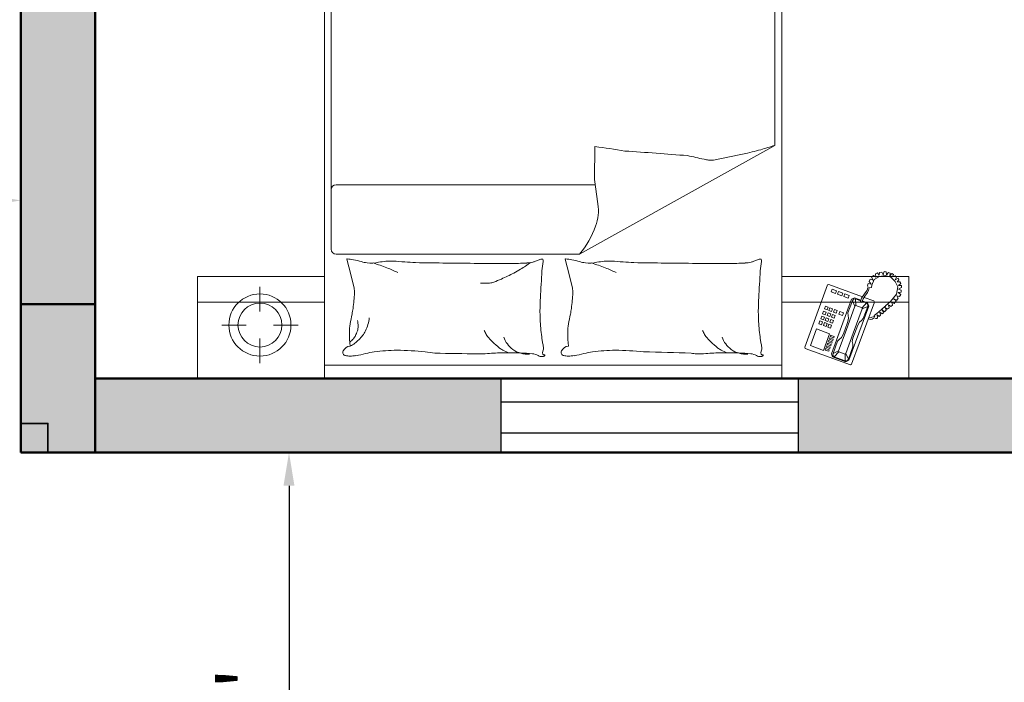
# Model space of a CAD drawing. Units: inches. Extents: x -7 to 1228, y -146 to 1091.
# Tile 3 of 88: x 60 to 179, y 32 to 112. Entities that reach past the tile are written whole.
import ezdxf

# ---------------------------------------------------------------- set-up
doc = ezdxf.new("R2010")
doc.units = ezdxf.units.IN
for name, color, linetype, lineweight in [('A-ANNO-DIMS', 2, 'Continuous', 18), ('A-COLS', 6, 'Continuous', 35), ('A-FURN', 8, 'Continuous', 18), ('A-GLAZ', 175, 'Continuous', 25), ('A-WALL', 7, 'Continuous', 50), ('A-WALL-PATT', 251, 'Continuous', 13)]:
    doc.layers.add(name, color=color, linetype=linetype, lineweight=lineweight)
doc.styles.add('DIM_FONT', font='SIMPLEX.shx', dxfattribs={"width": 0.8})
doc.styles.get("Standard").update_dxf_attribs({"font": 'arial.ttf'})
doc.dimstyles.new('ISO-25', dxfattribs={"dimtxt": 7, "dimasz": 4, "dimexe": 1.25, "dimexo": 0.625, "dimtad": 1, "dimdec": 1, "dimlunit": 3, "dimtxsty": 'Standard', "dimcen": 2.5, "dimadec": 0, "dimazin": 0, "dimtfac": 1, "dimtdec": 1, "dimtmove": 1, "dimatfit": 3, "dimfxl": 1, "dimarcsym": 0})

# ---------------------------------------------------------------- blocks, each defined once
blk = doc.blocks.new('A$C4F634EDD')
for p, q in [((0, 2.6295), (0, 2.2295)), ((0.5, 2.6295), (0, 2.6295)), ((0.5, 2.6295), (2.3, 2.6295)), ((0.5, 0.5295), (0.5, 2.6295)), ((0.5, 2.2295), (0.5, 2.6295)), ((2.3, 2.6295), (2.3, 0.5295)), ((2.3, 2.6295), (2.8, 2.6295)), ((2.3, 2.2295), (2.3, 2.6295)), ((2.8, 2.6295), (2.8, 2.2295)), ((0.2457, 2.5697), (0.2457, 2.4733)), ((0.5, 2.5771), (2.3, 2.5771)), ((2.392, 2.5115), (2.5692, 2.5765)), ((2.4985, 2.5445), (2.5516, 2.564)), ((2.5062, 2.5454), (2.5487, 2.561)), ((2.5483, 2.5347), (2.5487, 2.561)), ((2.5487, 2.561), (2.5571, 2.56)), ((2.5516, 2.564), (2.5637, 2.5584)), ((2.5571, 2.56), (2.5615, 2.5536)), ((2.5637, 2.5584), (2.6418, 2.3458)), ((2.5692, 2.5765), (2.574, 2.5743)), ((2.574, 2.5743), (2.6638, 2.3298)), ((2.412, 2.5007), (2.4634, 2.5196)), ((2.4634, 2.5196), (2.4875, 2.454)), ((2.4842, 2.5232), (2.47, 2.518)), ((2.4862, 2.5179), (2.4842, 2.5232)), ((2.4946, 2.5331), (2.4985, 2.5445)), ((2.5734, 2.3187), (2.4946, 2.5331)), ((2.5062, 2.5454), (2.5004, 2.5392)), ((2.5004, 2.5392), (2.5013, 2.5315)), ((2.5013, 2.5315), (2.5188, 2.4836)), ((2.5013, 2.5315), (2.5231, 2.5214)), ((2.5235, 2.5256), (2.5062, 2.5454)), ((2.5231, 2.5214), (2.5235, 2.5256)), ((2.5523, 2.4417), (2.5231, 2.5214)), ((2.5483, 2.5347), (2.5235, 2.5256)), ((2.5514, 2.5318), (2.5483, 2.5347)), ((2.5615, 2.5536), (2.5514, 2.5318)), ((2.5807, 2.4521), (2.5514, 2.5318)), ((2.5615, 2.5536), (2.5791, 2.5058)), ((2.3898, 2.5066), (2.392, 2.5115)), ((2.4795, 2.2621), (2.3898, 2.5066)), ((2.4361, 2.4352), (2.412, 2.5007)), ((2.47, 2.518), (2.472, 2.5127)), ((2.472, 2.5127), (2.4862, 2.5179)), ((2.4881, 2.5126), (2.4739, 2.5074)), ((2.4739, 2.5074), (2.4759, 2.502)), ((2.4759, 2.502), (2.4901, 2.5073)), ((2.492, 2.5019), (2.4778, 2.4967)), ((2.4778, 2.4967), (2.4798, 2.4914)), ((2.4798, 2.4914), (2.494, 2.4966)), ((2.4959, 2.4913), (2.4817, 2.4861)), ((2.4817, 2.4861), (2.4837, 2.4808)), ((2.4837, 2.4808), (2.4979, 2.486)), ((2.4998, 2.4807), (2.4856, 2.4755)), ((2.4901, 2.5073), (2.4881, 2.5126)), ((2.494, 2.4966), (2.492, 2.5019)), ((2.4979, 2.486), (2.4959, 2.4913)), ((2.5018, 2.4754), (2.4998, 2.4807)), ((2.5188, 2.4836), (2.5256, 2.4761)), ((2.5788, 2.4956), (2.5767, 2.4848)), ((2.5767, 2.4848), (2.5795, 2.4717)), ((2.5791, 2.5058), (2.5788, 2.4956)), ((2.4875, 2.454), (2.4361, 2.4352)), ((2.4856, 2.4755), (2.4876, 2.4702)), ((2.4876, 2.4702), (2.5018, 2.4754)), ((2.5037, 2.47), (2.4895, 2.4648)), ((2.4895, 2.4648), (2.4915, 2.4595)), ((2.4915, 2.4595), (2.5057, 2.4647)), ((2.5057, 2.4647), (2.5037, 2.47)), ((2.5256, 2.4761), (2.5342, 2.4692)), ((2.5342, 2.4692), (2.5405, 2.4574)), ((2.5405, 2.4574), (2.547, 2.4397)), ((2.5523, 2.4417), (2.5875, 2.346)), ((2.5795, 2.4717), (2.586, 2.454)), ((2.5807, 2.4521), (2.6158, 2.3564)), ((2.5984, 2.4204), (2.586, 2.454)), ((0.0957, 2.4197), (0.192, 2.4197)), ((0.2994, 2.4197), (0.3957, 2.4197)), ((2.4457, 2.4146), (2.4563, 2.4185)), ((2.4496, 2.4039), (2.4457, 2.4146)), ((2.4602, 2.4078), (2.4496, 2.4039)), ((2.4563, 2.4185), (2.4602, 2.4078)), ((2.4634, 2.4211), (2.474, 2.425)), ((2.4673, 2.4104), (2.4634, 2.4211)), ((2.4779, 2.4143), (2.4673, 2.4104)), ((2.4706, 2.4016), (2.4812, 2.4055)), ((2.474, 2.425), (2.4779, 2.4143)), ((2.4811, 2.4276), (2.4917, 2.4315)), ((2.485, 2.4169), (2.4811, 2.4276)), ((2.4812, 2.4055), (2.4851, 2.3949)), ((2.4956, 2.4208), (2.485, 2.4169)), ((2.4883, 2.4081), (2.4989, 2.412)), ((2.4922, 2.3975), (2.4883, 2.4081)), ((2.4917, 2.4315), (2.4956, 2.4208)), ((2.4989, 2.412), (2.5028, 2.4014)), ((2.5594, 2.4061), (2.547, 2.4397)), ((2.5622, 2.393), (2.5594, 2.4061)), ((2.6047, 2.4086), (2.5984, 2.4204)), ((2.6133, 2.4017), (2.6047, 2.4086)), ((0.2457, 2.366), (0.2457, 2.2697)), ((2.4528, 2.3951), (2.4635, 2.399)), ((2.4567, 2.3844), (2.4528, 2.3951)), ((2.4674, 2.3883), (2.4567, 2.3844)), ((2.46, 2.3756), (2.4706, 2.3795)), ((2.4639, 2.365), (2.46, 2.3756)), ((2.4635, 2.399), (2.4674, 2.3883)), ((2.4745, 2.3689), (2.4639, 2.365)), ((2.4745, 2.3909), (2.4706, 2.4016)), ((2.4706, 2.3795), (2.4745, 2.3689)), ((2.4851, 2.3949), (2.4745, 2.3909)), ((2.4777, 2.3821), (2.4883, 2.386)), ((2.4816, 2.3715), (2.4777, 2.3821)), ((2.4922, 2.3754), (2.4816, 2.3715)), ((2.4849, 2.3626), (2.4955, 2.3665)), ((2.4883, 2.386), (2.4922, 2.3754)), ((2.5028, 2.4014), (2.4922, 2.3975)), ((2.4954, 2.3886), (2.5061, 2.3925)), ((2.4993, 2.378), (2.4954, 2.3886)), ((2.4955, 2.3665), (2.4994, 2.3559)), ((2.51, 2.3819), (2.4993, 2.378)), ((2.5026, 2.3691), (2.5132, 2.373)), ((2.5065, 2.3585), (2.5026, 2.3691)), ((2.5061, 2.3925), (2.51, 2.3819)), ((2.5132, 2.373), (2.5171, 2.3624)), ((2.5238, 2.3769), (2.538, 2.3821)), ((2.5277, 2.3663), (2.5238, 2.3769)), ((2.5419, 2.3715), (2.5277, 2.3663)), ((2.538, 2.3821), (2.5419, 2.3715)), ((2.5598, 2.372), (2.5601, 2.3822)), ((2.5774, 2.3242), (2.5598, 2.372)), ((2.5601, 2.3822), (2.5622, 2.393)), ((2.6201, 2.3941), (2.6133, 2.4017)), ((2.6376, 2.3463), (2.6201, 2.3941)), ((2.6499, 2.3979), (2.6397, 2.3953)), ((2.6417, 2.39), (2.6488, 2.391)), ((2.6488, 2.391), (2.6538, 2.3895)), ((2.6551, 2.397), (2.6499, 2.3979)), ((2.6538, 2.3895), (2.6596, 2.388)), ((2.6627, 2.392), (2.6551, 2.397)), ((2.6596, 2.388), (2.6626, 2.3867)), ((2.6626, 2.3867), (2.6662, 2.388)), ((2.6692, 2.394), (2.6627, 2.392)), ((2.6662, 2.388), (2.6632, 2.3828)), ((2.6632, 2.3828), (2.6736, 2.3744)), ((2.6736, 2.3944), (2.6692, 2.394)), ((2.6765, 2.391), (2.6736, 2.3944)), ((2.6736, 2.3744), (2.6922, 2.3593)), ((2.6742, 2.3795), (2.6765, 2.391)), ((2.6824, 2.3858), (2.6742, 2.3795)), ((2.6873, 2.3815), (2.6824, 2.3858)), ((2.6853, 2.369), (2.6873, 2.3815)), ((2.6946, 2.376), (2.6853, 2.369)), ((2.6995, 2.3713), (2.6946, 2.376)), ((2.695, 2.3603), (2.6995, 2.3713)), ((2.7031, 2.3682), (2.695, 2.3603)), ((2.7096, 2.3616), (2.7031, 2.3682)), ((0, 2.3301), (0.5, 2.3301)), ((2.8, 2.3301), (2.3, 2.3301)), ((2.4672, 2.3561), (2.4778, 2.36)), ((2.4711, 2.3455), (2.4672, 2.3561)), ((2.4817, 2.3494), (2.4711, 2.3455)), ((2.4778, 2.36), (2.4817, 2.3494)), ((2.4888, 2.352), (2.4849, 2.3626)), ((2.4994, 2.3559), (2.4888, 2.352)), ((2.5171, 2.3624), (2.5065, 2.3585)), ((2.5774, 2.3242), (2.5875, 2.346)), ((2.5875, 2.346), (2.5905, 2.3431)), ((2.5905, 2.3431), (2.5901, 2.3168)), ((2.6154, 2.3522), (2.5905, 2.3431)), ((2.613, 2.3312), (2.6077, 2.3293)), ((2.6077, 2.3293), (2.6135, 2.3141)), ((2.6192, 2.3174), (2.613, 2.3312)), ((2.6153, 2.3261), (2.6327, 2.3324)), ((2.6158, 2.3564), (2.6154, 2.3522)), ((2.6154, 2.3522), (2.6327, 2.3324)), ((2.6376, 2.3463), (2.6158, 2.3564)), ((2.6369, 2.332), (2.6161, 2.3243)), ((2.6616, 2.3249), (2.6234, 2.3109)), ((2.6327, 2.3324), (2.6385, 2.3386)), ((2.6418, 2.3458), (2.6369, 2.332)), ((2.6385, 2.3386), (2.6376, 2.3463)), ((2.6638, 2.3298), (2.6616, 2.3249)), ((2.6922, 2.3593), (2.7051, 2.3473)), ((2.7051, 2.3473), (2.7079, 2.3475)), ((2.7062, 2.351), (2.7096, 2.3616)), ((2.7147, 2.3578), (2.7062, 2.351)), ((2.7079, 2.3475), (2.7079, 2.3443)), ((2.7079, 2.3443), (2.727, 2.3277)), ((2.7214, 2.3517), (2.7147, 2.3578)), ((2.7196, 2.34), (2.7214, 2.3517)), ((2.7286, 2.3466), (2.7196, 2.34)), ((2.727, 2.3277), (2.7512, 2.2983)), ((2.7346, 2.3423), (2.7286, 2.3466)), ((2.732, 2.3295), (2.7346, 2.3423)), ((2.7423, 2.3345), (2.732, 2.3295)), ((2.7406, 2.3172), (2.7495, 2.325)), ((2.7495, 2.325), (2.7423, 2.3345)), ((2.6172, 2.3086), (2.4844, 2.2599)), ((2.5114, 2.2959), (2.4936, 2.2894)), ((2.4936, 2.2894), (2.4976, 2.2788)), ((2.5153, 2.2853), (2.5114, 2.2959)), ((2.5362, 2.305), (2.5185, 2.2985)), ((2.5185, 2.2985), (2.5224, 2.2879)), ((2.5224, 2.2879), (2.5401, 2.2944)), ((2.5401, 2.2944), (2.5362, 2.305)), ((2.561, 2.3141), (2.5433, 2.3076)), ((2.5433, 2.3076), (2.5472, 2.297)), ((2.5472, 2.297), (2.5649, 2.3035)), ((2.5649, 2.3035), (2.561, 2.3141)), ((2.5855, 2.3131), (2.5734, 2.3187)), ((2.5818, 2.3178), (2.5774, 2.3242)), ((2.5901, 2.3168), (2.5818, 2.3178)), ((2.6104, 2.3222), (2.5855, 2.3131)), ((2.5901, 2.3168), (2.6097, 2.324)), ((2.6135, 2.3141), (2.6244, 2.2977)), ((2.626, 2.3069), (2.6192, 2.3174)), ((2.6244, 2.2977), (2.6349, 2.2825)), ((2.6365, 2.2916), (2.626, 2.3069)), ((2.6407, 2.2834), (2.6365, 2.2916)), ((2.7519, 2.3218), (2.7406, 2.3172)), ((2.7512, 2.2983), (2.756, 2.2695)), ((2.7575, 2.3144), (2.7519, 2.3218)), ((2.7526, 2.3045), (2.7575, 2.3144)), ((2.7622, 2.308), (2.7526, 2.3045)), ((2.7574, 2.2924), (2.7673, 2.2997)), ((2.7687, 2.2905), (2.7574, 2.2924)), ((2.7673, 2.2997), (2.7622, 2.308)), ((2.7699, 2.2828), (2.7687, 2.2905)), ((0.5953, 2.1912), (0.616, 2.2738)), ((1.4546, 2.1912), (1.4752, 2.2738)), ((2.4844, 2.2599), (2.4795, 2.2621)), ((2.4976, 2.2788), (2.5153, 2.2853)), ((2.6349, 2.2825), (2.638, 2.273)), ((2.6399, 2.2712), (2.6374, 2.2659)), ((2.6374, 2.2659), (2.6398, 2.257)), ((2.638, 2.273), (2.6399, 2.2712)), ((2.6398, 2.257), (2.6509, 2.259)), ((2.6438, 2.2739), (2.6407, 2.2834)), ((2.6509, 2.259), (2.6431, 2.2492)), ((2.6431, 2.2492), (2.6473, 2.2398)), ((2.6519, 2.2716), (2.6438, 2.2739)), ((2.6535, 2.2628), (2.6519, 2.2716)), ((2.6636, 2.2409), (2.6535, 2.2628)), ((2.7459, 2.2483), (2.7284, 2.2317)), ((2.756, 2.2695), (2.7459, 2.2483)), ((2.7529, 2.2505), (2.7645, 2.2498)), ((2.7607, 2.2424), (2.7529, 2.2505)), ((2.7587, 2.279), (2.7699, 2.2828)), ((2.7708, 2.2725), (2.7587, 2.279)), ((2.759, 2.2637), (2.7706, 2.2643)), ((2.7676, 2.2559), (2.759, 2.2637)), ((2.7645, 2.2498), (2.7676, 2.2559)), ((2.7706, 2.2643), (2.7708, 2.2725)), ((0, 2.2295), (0.5, 2.2295)), ((2.8, 2.2295), (2.3, 2.2295)), ((2.6473, 2.2398), (2.6592, 2.2429)), ((2.6592, 2.2429), (2.6521, 2.2314)), ((2.6521, 2.2314), (2.6598, 2.2248)), ((2.6598, 2.2248), (2.6697, 2.2309)), ((2.6836, 2.2287), (2.6636, 2.2409)), ((2.6697, 2.2309), (2.6684, 2.219)), ((2.6684, 2.219), (2.6761, 2.2145)), ((2.6761, 2.2145), (2.6821, 2.2237)), ((2.6821, 2.2237), (2.6843, 2.2135)), ((2.7063, 2.2256), (2.6836, 2.2287)), ((2.6843, 2.2135), (2.6927, 2.2117)), ((2.6927, 2.2117), (2.6986, 2.222)), ((2.6986, 2.222), (2.7019, 2.2098)), ((2.7019, 2.2098), (2.7102, 2.2104)), ((2.7284, 2.2317), (2.7063, 2.2256)), ((2.7102, 2.2104), (2.7113, 2.2218)), ((2.7113, 2.2218), (2.7192, 2.2137)), ((2.7192, 2.2137), (2.7255, 2.2152)), ((2.7255, 2.2152), (2.7242, 2.2265)), ((2.7242, 2.2265), (2.7324, 2.2165)), ((2.7324, 2.2165), (2.7386, 2.2208)), ((2.7386, 2.2208), (2.7354, 2.2306)), ((2.7354, 2.2306), (2.7462, 2.2264)), ((2.7509, 2.2314), (2.7459, 2.2418)), ((2.7459, 2.2418), (2.7568, 2.2352)), ((2.7462, 2.2264), (2.7509, 2.2314)), ((2.7568, 2.2352), (2.7607, 2.2424)), ((0.5878, 2.1612), (0.5953, 2.1912)), ((1.4471, 2.1612), (1.4546, 2.1912)), ((1.5035, 2.141), (0.5458, 2.141)), ((1.5035, 2.141), (2.2716, 1.7136)), ((0.5258, 2.121), (0.5258, 0.5617)), ((1.576, 1.9433), (1.5624, 1.8479)), ((0.5458, 1.8684), (1.5653, 1.8684)), ((1.5624, 1.8479), (1.5641, 1.7178)), ((2.2716, 0.5617), (2.2716, 1.7136))]:
    blk.add_line(p, q)
for radius in [0.1222, 0.0865]:
    blk.add_circle((0.2457, 2.4197), radius)
for centre, radius, start, end in [((0.5848, 2.5274), 0.0131, 101.2724, 206.5805), ((0.6036, 2.5368), 0.0342, 206.5805, 265.5998), ((0.5999, 2.4516), 0.0904, 90, 101.2724), ((0.5999, 2.3808), 0.1611, 81.5628, 90), ((0.5788, 2.2388), 0.3048, 74.256, 81.5628), ((0.7272, 2.7653), 0.2422, 254.256, 262.4531), ((0.7851, 3.2019), 0.6827, 262.4531, 270), ((0.7851, 3.5682), 1.049, 270, 276.0867), ((0.8402, 3.0514), 0.5293, 276.0867, 280.1899), ((1.1602, -8.1346), 10.6675, 90.30153, 91.21582), ((1.1169, 2.2433), 0.2897, 85.1982, 92.5386), ((1.2142, 3.4021), 0.8732, 265.1982, 269.4243), ((1.3082, 2.3102), 0.234, 110.8603, 117.2396), ((1.2204, 4.0232), 1.4943, 269.4243, 271.9079), ((1.2995, 2.4357), 0.0992, 105.9352, 126.0864), ((1.2429, 3.3501), 0.8208, 271.9079, 275.2592), ((1.2995, 2.4357), 0.0992, 85.7841, 105.9352), ((1.3132, 2.5864), 0.0539, 275.2592, 300.6513), ((1.3554, 2.5152), 0.0289, 85.6975, 120.6513), ((1.3556, 2.519), 0.0251, 68.2117, 85.6975), ((1.3739, 2.5288), 0.0156, 158.0096, 201.421), ((1.3634, 2.533), 0.00428, 78.1069, 158.0096), ((1.3288, 2.5111), 0.0328, 351.8665, 21.421), ((1.3647, 2.5395), 0.00232, 258.1069, 19.564), ((1.3637, 2.5391), 0.00342, 19.564, 68.2117), ((1.444, 2.5274), 0.0131, 101.2724, 206.5805), ((1.4628, 2.5368), 0.0342, 206.5805, 265.5998), ((1.4591, 2.4516), 0.0904, 90, 101.2724), ((1.4591, 2.3808), 0.1611, 81.5628, 90), ((1.438, 2.2388), 0.3048, 74.256, 81.5628), ((1.5865, 2.7653), 0.2422, 254.256, 262.4531), ((1.6443, 3.2019), 0.6827, 262.4531, 270), ((1.6443, 3.5682), 1.049, 270, 276.0867), ((1.4785, 15.4878), 12.9656, 271.22425, 272.05324), ((1.97, 2.3805), 0.1524, 92.5386, 100.1899), ((1.9761, 2.2433), 0.2897, 85.1982, 92.5386), ((2.0734, 3.4021), 0.8732, 265.1982, 269.4243), ((2.1674, 2.3102), 0.234, 110.8603, 117.2396), ((2.0797, 4.0232), 1.4943, 269.4243, 271.9079), ((2.1588, 2.4357), 0.0992, 105.9352, 126.0864), ((2.1021, 3.3501), 0.8208, 271.9079, 275.2592), ((2.1588, 2.4357), 0.0992, 85.7841, 105.9352), ((2.1724, 2.5864), 0.0539, 275.2592, 300.6513), ((2.2146, 2.5152), 0.0289, 85.6975, 120.6513), ((2.2149, 2.519), 0.0251, 68.2117, 85.6975), ((2.2331, 2.5288), 0.0156, 158.0096, 201.421), ((2.2226, 2.533), 0.00428, 78.1069, 158.0096), ((2.1881, 2.5111), 0.0328, 351.8665, 21.421), ((2.224, 2.5395), 0.00232, 258.1069, 19.564), ((2.2229, 2.5391), 0.00342, 19.564, 68.2117), ((1.0898, 2.4496), 0.4918, 173.7676, 180), ((0.5462, 2.4142), 0.0899, 41.4429, 53.7359), ((0.5368, 2.3783), 0.1399, 45.0976, 62.7964), ((1.3165, 2.3233), 0.2252, 133.8115, 140.9651), ((1.4317, 2.2032), 0.3916, 128.3886, 133.8115), ((1.2362, 2.45), 0.0768, 117.2396, 128.3886), ((1.2995, 2.4357), 0.0992, 143.8234, 161.5603), ((1.2995, 2.4357), 0.0992, 126.0864, 143.8234), ((1.5522, 2.448), 0.1983, 167.8905, 172.3191), ((1.1177, 2.5413), 0.246, 347.8905, 351.8665), ((1.949, 2.4496), 0.4918, 173.7676, 180), ((2.1757, 2.3233), 0.2252, 133.8115, 140.9651), ((2.291, 2.2032), 0.3916, 128.3886, 133.8115), ((2.0954, 2.45), 0.0768, 117.2396, 128.3886), ((2.1588, 2.4357), 0.0992, 143.8234, 161.5603), ((2.1588, 2.4357), 0.0992, 126.0864, 143.8234), ((2.4114, 2.448), 0.1983, 167.8905, 172.3191), ((1.977, 2.5413), 0.246, 347.8905, 351.8665), ((0.8019, 2.4496), 0.204, 180, 189.6844), ((0.5741, 2.4389), 0.0526, 25.3551, 41.4429), ((0.4851, 2.3967), 0.1511, 21.8149, 25.3551), ((0.4345, 2.3765), 0.2056, 18.7799, 21.8149), ((0.576, 2.4246), 0.0562, 0, 18.7799), ((0.5368, 2.3783), 0.1399, 27.3988, 45.0976), ((0.5368, 2.3783), 0.1399, 16.515, 27.3988), ((1.3127, 2.3625), 0.2002, 151.6832, 156.9972), ((1.1799, 2.4341), 0.0493, 140.9651, 151.6832), ((2.2605, 2.3525), 0.9131, 172.3191, 176.6313), ((1.6611, 2.4496), 0.204, 180, 189.6844), ((2.1719, 2.3625), 0.2002, 151.6832, 156.9972), ((2.0391, 2.4341), 0.0493, 140.9651, 151.6832), ((3.1198, 2.3525), 0.9131, 172.3191, 176.6313), ((1.4703, 2.5637), 0.882, 189.6844, 192.1984), ((0.5406, 2.4246), 0.0915, 345.3149, 0), ((0.5368, 2.3783), 0.1399, 5.6311, 16.515), ((2.0266, 2.3663), 0.6787, 176.6313, 181.6331), ((2.3295, 2.5637), 0.882, 189.6844, 192.1984), ((2.8858, 2.3663), 0.6787, 176.6313, 181.6331), ((0.2982, 2.3103), 0.3171, 8.0051, 12.1984), ((1.1575, 2.3103), 0.3171, 8.0051, 12.1984), ((-0.0401, 2.2627), 0.6588, 2.6649, 8.0051), ((2.7128, 2.3859), 1.3652, 181.6331, 183.055), ((0.8191, 2.2627), 0.6588, 2.6649, 8.0051), ((3.5721, 2.3859), 1.3652, 181.6331, 183.055), ((0.5503, 2.2902), 0.0677, 345.9548, 2.6649), ((14.9657, 3.0398), 13.6356, 183.05496, 183.50486), ((1.4096, 2.2902), 0.0677, 345.9548, 2.6649), ((15.8249, 3.0398), 13.6356, 183.05496, 183.50486), ((1.1303, 1.9835), 0.2721, 85.9172, 93.5552), ((1.1455, 2.197), 0.058, 69.3257, 85.9172), ((0.9871, 1.7772), 0.5066, 65.6735, 69.3257), ((0.473, 2.8815), 0.7387, 293.4844, 295.3111), ((0.6058, 0.9338), 1.4323, 63.5015, 65.6735), ((1.1054, 1.9358), 0.3126, 57.865, 63.5015), ((1.3322, 2.8815), 0.7387, 293.4844, 295.3111), ((0.5763, 2.3896), 0.2297, 279.4841, 287.3864), ((0.6807, 2.0561), 0.1197, 96.4341, 107.3864), ((0.6836, 2.0301), 0.1459, 78.4414, 96.4341), ((0.473, 2.8815), 0.7387, 287.1982, 289.428), ((0.759, 2.3985), 0.2301, 258.4414, 272.7491), ((0.473, 2.8815), 0.7387, 289.428, 291.6577), ((0.473, 2.8815), 0.7387, 291.6577, 293.4844), ((0.7026, 3.5718), 1.4048, 272.7491, 274.6176), ((0.9136, 0.9591), 1.2165, 92.6096, 94.6176), ((1.2501, -19.8405), 22.0183, 90.37908, 91.01965), ((1.2012, -3.5404), 5.7185, 89.7135, 90.9704), ((1.224, 1.0141), 1.164, 86.426, 89.7135), ((0.8841, 1.5835), 0.7286, 54.1737, 57.865), ((1.2875, 2.0302), 0.1459, 77.131, 86.426), ((1.3099, 2.1283), 0.0453, 62.7159, 77.131), ((1.6762, 2.2258), 0.3212, 183.5049, 189.9984), ((1.3409, 2.1667), 0.0193, 343.3022, 9.9984), ((1.4355, 2.3896), 0.2297, 279.4841, 287.3864), ((1.5399, 2.0561), 0.1197, 96.4341, 107.3864), ((1.5429, 2.0301), 0.1459, 78.4414, 96.4341), ((1.3322, 2.8815), 0.7387, 287.1982, 289.428), ((1.6182, 2.3985), 0.2301, 258.4414, 272.7491), ((1.3322, 2.8815), 0.7387, 289.428, 291.6577), ((1.3322, 2.8815), 0.7387, 291.6577, 293.4844), ((1.5619, 3.5718), 1.4048, 272.7491, 274.6176), ((1.7729, 0.9591), 1.2165, 92.6096, 94.6176), ((2.1093, -19.8405), 22.0183, 90.37908, 91.01965), ((2.0605, -3.5404), 5.7185, 89.7135, 90.9704), ((2.0833, 1.0141), 1.164, 86.426, 89.7135), ((2.1467, 2.0302), 0.1459, 77.131, 86.426), ((2.1691, 2.1283), 0.0453, 62.7159, 77.131), ((2.5355, 2.2258), 0.3212, 183.5049, 189.9984), ((2.2001, 2.1667), 0.0193, 343.3022, 9.9984), ((0.5458, 2.121), 0.02, 90, 180), ((0.5887, 2.1609), 0.000917, 165.9551, 274.0829), ((0.5695, 2.4301), 0.2708, 274.0829, 279.4841), ((1.3658, 2.2367), 0.0767, 242.7159, 253.7788), ((1.3688, 2.247), 0.0875, 253.7788, 262.8796), ((1.3581, 2.1615), 0.00132, 262.8796, 343.3022), ((1.448, 2.1609), 0.000917, 165.9551, 274.0829), ((1.4288, 2.4301), 0.2708, 274.0829, 279.4841), ((1.2147, 1.9017), 0.3751, 20.1488, 39.6445), ((2.2251, 2.2367), 0.0767, 242.7159, 253.7788), ((2.2281, 2.247), 0.0875, 253.7788, 262.8796), ((2.2174, 2.1615), 0.00132, 262.8796, 343.3022), ((1.3977, 1.9688), 0.1801, 351.8644, 20.1488), ((0.5458, 1.8884), 0.02, 180, 270), ((0.6102, 18.0525), 16.3521, 273.75703, 274.62393), ((1.4194, 4.2174), 2.5158, 281.6741, 283.1904), ((2.0378, 1.5789), 0.1942, 97.7304, 103.1904), ((2.0195, 1.7137), 0.0581, 79.2724, 97.7304), ((1.2737, -2.2227), 4.0646, 77.0745, 79.2724), ((1.0582, 5.4638), 3.7801, 277.692, 279.495), ((2.0359, 1.0981), 0.6574, 74.0648, 77.0745), ((1.7125, -0.0344), 1.8351, 72.2636, 74.0648)]:
    blk.add_arc(centre, radius, start, end)
at = {"style": 'DIM_FONT', "width": 0.8, "flags": 9}
for tag, p in [('YSIZE', (0.5, 2.6295)), ('XSIZE', (0.5, 2.6295)), ('XSIZE', (2.2985, 2.6295)), ('YSIZE', (2.2985, 2.6295))]:
    blk.add_attdef(tag, p, '', height=0.0005, dxfattribs=at)
blk = doc.blocks.new('*D9')
at = {"layer": 'A-ANNO-DIMS', "color": 0, "lineweight": -2, "transparency": 16777216}
for p, q in [((92.31, 60), (91.25, 60)), ((92.5, 56), (92.5, 4)), ((92.31, 0), (91.25, 0))]:
    blk.add_line(p, q, dxfattribs=at)
at = {"layer": 'A-ANNO-DIMS', "color": 0, "transparency": 16777216}
for points in [[(91.83, 56), (93.16, 56), (92.5, 60)], [(91.83, 4), (93.16, 4), (92.5, 0)]]:
    blk.add_solid(points, dxfattribs=at)
at = {"layer": 'Defpoints', "color": 0, "transparency": 16777216}
for p in [(92.94, 60), (92.94, 0), (92.5, 0)]:
    blk.add_point(p, dxfattribs=at)
at = {"layer": 'A-ANNO-DIMS', "color": 0, "transparency": 16777216, "insert": (88.31, 30), "char_height": 7, "attachment_point": 5, "rotation": 90}
blk.add_mtext("5'", dxfattribs=at)
blk = doc.blocks.new('*D10')
at = {"layer": 'A-ANNO-DIMS', "color": 0, "lineweight": -2, "transparency": 16777216}
for p, q in [((0, 96.81), (0, 89.3)), ((60, 96.81), (60, 89.3)), ((56, 90.55), (4, 90.55))]:
    blk.add_line(p, q, dxfattribs=at)
at = {"layer": 'A-ANNO-DIMS', "color": 0, "transparency": 16777216}
for points in [[(4, 91.22), (4, 89.88), (0, 90.55)], [(56, 91.22), (56, 89.88), (60, 90.55)]]:
    blk.add_solid(points, dxfattribs=at)
at = {"layer": 'Defpoints', "color": 0, "transparency": 16777216}
for p in [(0, 97.43), (60, 97.43), (0, 90.55)]:
    blk.add_point(p, dxfattribs=at)
at = {"layer": 'A-ANNO-DIMS', "color": 0, "transparency": 16777216, "insert": (30, 94.74), "char_height": 7, "attachment_point": 5}
blk.add_mtext("5'", dxfattribs=at)
blk = doc.blocks.new('WIN-36')
for p, q in [((0, 36), (0, 0)), ((9, 36), (0, 36)), ((2.34, 36), (2.34, 0)), ((6.14, 0), (6.14, 36)), ((9, 0), (9, 36)), ((0, 0), (9, 0)), ((2.34, 0), (6.14, 0))]:
    blk.add_line(p, q)

msp = doc.modelspace()

# ---------------------------------------------------------------- hatches: boundary and pattern name
at = {"layer": 'A-COLS'}
h = msp.add_hatch(color=256, dxfattribs=at)
h.dxf.hatch_style = 1
h.paths.add_polyline_path([(60, 63.55), (63.29, 63.55), (63.29, 60), (69, 60), (69, 78), (60, 78)])
h = msp.add_hatch(color=256, dxfattribs=at)
h.dxf.hatch_style = 1
h.paths.add_polyline_path([(60, 63.55), (60, 60), (63.29, 60), (63.29, 63.55)])
at = {"layer": 'A-WALL-PATT'}
h = msp.add_hatch(color=256, dxfattribs=at)
h.dxf.hatch_style = 1
h.paths.add_polyline_path([(69, 568), (60, 568), (60, 493), (63.29, 493), (69, 493)])
h.paths.add_polyline_path([(69, 662.41), (60, 662.41), (60, 586), (69, 586)], flags=17)
h.paths.add_polyline_path([(69, 723), (184, 723), (184, 734), (179, 734), (179, 728), (69, 728), (69, 741.62), (60, 741.62), (60, 698.41), (69, 698.41)], flags=17)
h.paths.add_polyline_path([(69, 782), (231, 782), (231, 728), (231, 723), (231, 586), (236, 586), (236, 787), (69, 787), (69, 800.13), (60, 800.13), (60, 765.62), (69, 765.62)])
h.paths.add_polyline_path([(184, 842), (189, 842), (189, 848), (173, 848), (173, 842), (179, 842), (179, 787), (184, 787)])
h.paths.add_polyline_path([(118.22, 69), (69, 69), (69, 60), (118.22, 60)])
h.paths.add_polyline_path([(227, 69), (154.22, 69), (154.22, 60), (227, 60)])
h.paths.add_polyline_path([(236, 60), (232.71, 60), (227, 60), (227, 36), (236, 36)])
h.paths.add_polyline_path([(389, 60), (380, 60), (380, 36), (389, 36)])
h.paths.add_polyline_path([(384, 181), (380, 181), (380, 115), (380, 78), (384, 78)])
h.paths.add_polyline_path([(380, 115), (334.55, 115), (334.55, 109), (380, 109)])
h.paths.add_polyline_path([(274.55, 115), (236, 115), (236, 201), (232.71, 201), (231, 201), (231, 78), (236, 78), (236, 109), (274.55, 109)])
h.paths.add_polyline_path([(69, 123), (60, 123), (60, 78), (69, 78)])
h.paths.add_polyline_path([(69, 201), (60, 201), (60, 159), (69, 159)])
h.paths.add_polyline_path([(143, 219), (69, 219), (69, 213), (143, 213)], flags=17)
h.paths.add_polyline_path([(189, 219), (184, 219), (184, 274), (231, 274), (231, 219), (236, 219), (236, 279), (184, 279), (184, 297), (179, 297), (179, 279), (69, 279), (69, 290.91), (60, 290.91), (60, 262.18), (69, 262.18), (69, 274), (179, 274), (179, 219), (173, 219), (173, 213), (189, 213)])
h.paths.add_polyline_path([(69, 238.18), (60, 238.18), (60, 219), (69, 219)], flags=17)
h.paths.add_polyline_path([(69, 333), (60, 333), (60, 314.91), (69, 314.91), (69, 316.96)])
h.paths.add_polyline_path([(190, 338), (184, 338), (69, 338), (69, 333), (179, 333), (179, 327), (184, 327), (184, 333.02), (190, 333.05)])
h.paths.add_polyline_path([(69, 386.81), (60, 386.81), (60, 351), (69, 351)])
h.paths.add_polyline_path([(69, 475), (60, 475), (60, 422.81), (69, 422.81)])
h.paths.add_polyline_path([(236, 475), (231, 475), (231, 351.24), (236, 351.24)])
h.paths.add_polyline_path([(384, 475), (380, 475), (380, 362), (384, 362)])
h.paths.add_polyline_path([(547, 307), (439, 307), (439, 356), (445, 356), (445, 362), (433, 362), (433, 307), (380, 307), (380, 244), (380, 241), (384, 241), (384, 301), (433, 301), (433, 277), (439, 277), (439, 301), (547, 301)])
h.paths.add_polyline_path([(547, 241), (439, 241), (439, 247), (433, 247), (433, 235), (547, 235)])
h.paths.add_polyline_path([(450, 69), (440.29, 69), (424.89, 69), (389, 69), (389, 60), (450, 60)])
h.paths.add_polyline_path([(547, 69), (486, 69), (486, 60), (547, 60)])
h.paths.add_polyline_path([(556, 148.27), (547, 148.27), (547, 78), (556, 78)])
h.paths.add_polyline_path([(556, 223), (547, 223), (547, 195), (547, 184.27), (556, 184.27)])
h.paths.add_polyline_path([(556, 311.19), (547, 311.19), (547, 273.08), (556, 273.08)])
h.paths.add_polyline_path([(556, 344), (552.71, 344), (547, 344), (547, 335.19), (556, 335.19)])
h.paths.add_polyline_path([(556, 249.08), (547, 249.08), (547, 241), (556, 241)])
h.paths.add_polyline_path([(547, 362), (475, 362), (475, 356), (547, 356)], flags=0)
h.paths.add_polyline_path([(556, 399.62), (547, 399.62), (547, 362), (556, 362)])
h.paths.add_polyline_path([(556, 475), (547, 475), (547, 435.62), (556, 435.62)])
h.paths.add_polyline_path([(547, 493), (389, 493), (389, 487), (547, 487)])
h.paths.add_polyline_path([(380, 493), (278, 493), (278, 487), (380, 487)])
h.paths.add_polyline_path([(227, 493), (69, 493), (69, 487), (227, 487)])
h.paths.add_polyline_path([(643, 122.44), (634, 122.44), (634, 78), (643, 78)])
h.paths.add_polyline_path([(702.5, 69), (692.79, 69), (677.39, 69), (643, 69), (643, 60), (702.5, 60)])
h.paths.add_polyline_path([(798, 69), (738.5, 69), (738.5, 60), (798, 60)])
h.paths.add_polyline_path([(807, 60), (803.71, 60), (798, 60), (798, 36), (807, 36)])
h.paths.add_polyline_path([(807, 109), (846.75, 109), (846.75, 115), (807, 115), (807, 159), (802, 159), (802, 78), (807, 78)])
h.paths.add_polyline_path([(807, 201), (802, 201), (802, 195), (807, 195)])
h.paths.add_polyline_path([(643, 201), (634, 201), (634, 158.44), (643, 158.44)])
h.paths.add_polyline_path([(756, 225), (751, 225), (751, 219), (643, 219), (643, 213), (756, 213)])
h.paths.add_polyline_path([(643, 240.85), (634, 240.85), (634, 219), (643, 219)])
h.paths.add_polyline_path([(643, 274), (643, 288.63), (634, 288.63), (634, 264.85), (643, 264.85)])
h.paths.add_polyline_path([(802, 279), (756, 279), (756, 297), (751, 297), (751, 279), (643, 279), (643, 274), (751, 274), (751, 255), (756, 255), (756, 274), (802, 274)])
h.paths.add_polyline_path([(807, 333), (803.71, 333), (802, 333), (802, 279), (802, 274), (802, 219), (807, 219)])
h.paths.add_polyline_path([(956, 182), (951, 182), (951, 115), (906.75, 115), (906.75, 109), (951, 109), (951, 78), (956, 78)])
h.paths.add_polyline_path([(960, 60), (951, 60), (951, 36), (960, 36)])
h.paths.add_polyline_path([(1021, 69), (1005.78, 69), (960, 69), (960, 60), (1021, 60)])
h.paths.add_polyline_path([(956, 224), (951, 224), (951, 218), (956, 218)])
h.paths.add_polyline_path([(956, 302), (1004, 302), (1004, 278), (1010, 278), (1010, 302), (1118, 302), (1118, 290.81), (1127, 290.81), (1127, 326.97), (1118, 326.97), (1118, 320.97), (1118, 307), (1010, 307), (1010, 356), (1016, 356), (1016, 362), (1004, 362), (1004, 307), (951, 307), (951, 244), (951, 242), (954.29, 242), (956, 242)])
h.paths.add_polyline_path([(643, 333), (634, 333), (634, 312.63), (643, 312.63), (643, 316.96)])
h.paths.add_polyline_path([(756, 338), (643, 338), (643, 333), (751, 333), (751, 327), (756, 327)])
h.paths.add_polyline_path([(643, 388), (634, 388), (634, 351), (643, 351)])
h.paths.add_polyline_path([(807, 357), (802, 357), (802, 351), (807, 351)])
h.paths.add_polyline_path([(807, 475), (802, 475), (802, 393), (807, 393)])
h.paths.add_polyline_path([(643, 475), (634, 475), (634, 424), (643, 424)])
h.paths.add_polyline_path([(798, 493), (643, 493), (643, 487), (798, 487)])
h.paths.add_polyline_path([(634, 493), (556, 493), (556, 487), (634, 487)])
h.paths.add_polyline_path([(813, 493), (807, 493), (807, 487), (813, 487)])
h.paths.add_polyline_path([(951, 493), (849, 493), (849, 487), (951, 487)])
h.paths.add_polyline_path([(956, 484), (951, 484), (951, 374), (956, 374)])
h.paths.add_polyline_path([(1109, 493), (969, 493), (969, 487), (1109, 487)])
h.paths.add_polyline_path([(1127, 484), (1118, 484), (1118, 450.64), (1127, 450.64)])
h.paths.add_polyline_path([(1127, 414.64), (1118, 414.64), (1118, 365), (1127, 365)])
h.paths.add_polyline_path([(1109, 362), (1046, 362), (1046, 356), (1109, 356)], flags=17)
h.paths.add_polyline_path([(1127, 356), (1123.45, 356), (1118, 356), (1118, 350.97), (1127, 350.97)], flags=0)
h.paths.add_polyline_path([(1127, 266.81), (1118, 266.81), (1118, 262.36), (1118, 242), (1127, 242)], flags=17)
h.paths.add_polyline_path([(1118, 242), (1010, 242), (1010, 248), (1004, 248), (1004, 237), (1118, 237)])
h.paths.add_polyline_path([(1127, 224), (1118, 224), (1118, 170), (1127, 170)])
h.paths.add_polyline_path([(1127, 134), (1118, 134), (1118, 78), (1127, 78)])
h.paths.add_polyline_path([(1118, 69), (1057, 69), (1057, 60), (1118, 60)])
h.paths.add_polyline_path([(227, 571.55), (227, 574), (69, 574), (69, 568), (227, 568)])
h.paths.add_polyline_path([(380, 571.55), (380, 574), (278, 574), (278, 568), (380, 568)])
h.paths.add_polyline_path([(242, 574), (236, 574), (236, 568), (242, 568)])
h.paths.add_polyline_path([(547, 571.55), (547, 574), (389, 574), (389, 568), (547, 568)])
h.paths.add_polyline_path([(384, 733), (380, 733), (380, 586), (384, 586)])
h.paths.add_polyline_path([(556, 646), (634, 646), (634, 655), (547, 655), (547, 586), (556, 586)])
h.paths.add_polyline_path([(634, 574), (556, 574), (556, 568), (634, 568)])
h.paths.add_polyline_path([(643, 655), (634, 655), (634, 586), (643, 586)])
h.paths.add_polyline_path([(798, 574), (643, 574), (643, 568), (798, 568)])
h.paths.add_polyline_path([(643, 663.85), (634, 663.85), (634, 655), (643, 655)])
h.paths.add_polyline_path([(556, 676.97), (547, 676.97), (547, 655), (556, 655)])
h.paths.add_polyline_path([(556, 733), (547, 733), (547, 712.97), (556, 712.97)])
h.paths.add_polyline_path([(643, 710), (634, 710), (634, 699.85), (643, 699.85)])
h.paths.add_polyline_path([(807, 668), (802, 668), (802, 586), (807, 586)])
h.paths.add_polyline_path([(951, 574), (849, 574), (849, 568), (951, 568)])
h.paths.add_polyline_path([(956, 691), (951, 691), (951, 577), (956, 577)])
h.paths.add_polyline_path([(1109, 574), (969, 574), (969, 568), (1109, 568)])
h.paths.add_polyline_path([(1127, 643.4), (1118, 643.4), (1118, 577), (1127, 577)])
h.paths.add_polyline_path([(1127, 568), (1123.45, 568), (1118, 568), (1118, 493), (1127, 493)])
h.paths.add_polyline_path([(1127, 733), (1118, 733), (1118, 679.4), (1127, 679.4)])
h.paths.add_polyline_path([(1127, 777.35), (1118, 777.35), (1118, 770.04), (1118, 751), (1127, 751)], flags=17)
h.paths.add_polyline_path([(1118, 751), (1010, 751), (1010, 757), (1004, 757), (1004, 745), (1118, 745)])
h.paths.add_polyline_path([(956, 811), (1004, 811), (1004, 787), (1010, 787), (1010, 811), (1017.87, 811), (1017.87, 811.63, -0.414214), (1018.25, 812), (1031.98, 812, -0.414214), (1032.35, 811.63), (1032.35, 811), (1118, 811), (1118, 801.35), (1127, 801.35), (1127, 834.69), (1118, 834.69), (1118, 830.24), (1118, 817), (1010, 817), (1010, 866), (1016, 866), (1016, 872), (1004, 872), (1004, 817), (956, 817), (956, 866), (951, 866), (951, 751), (954.29, 751), (956, 751)])
h.paths.add_polyline_path([(1118, 872), (1046, 872), (1046, 866), (1118, 866)], flags=17)
h.paths.add_polyline_path([(1127, 924.71), (1118, 924.71), (1118, 884), (1127, 884)])
h.paths.add_polyline_path([(1127, 866), (1123.71, 866), (1118, 866), (1118, 858.69), (1127, 858.69)], flags=17)
h.paths.add_polyline_path([(956, 983), (951, 983), (951, 952), (807, 952), (807, 983), (802, 983), (802, 902), (807, 902), (807, 946), (951, 946), (951, 884), (956, 884)])
h.paths.add_polyline_path([(807, 842), (802, 842), (802, 787), (756, 787), (756, 806), (751, 806), (751, 787), (643, 787), (643, 782), (751, 782), (751, 764), (756, 764), (756, 782), (802, 782), (802, 728), (807, 728)])
h.paths.add_polyline_path([(756, 848), (643, 848), (643, 842), (751, 842), (751, 836), (756, 836)])
h.paths.add_polyline_path([(756, 734), (751, 734), (751, 728), (643, 728), (643, 723), (756, 723)])
h.paths.add_polyline_path([(643, 749.79), (634, 749.79), (634, 728), (637.29, 728), (643, 728)])
h.paths.add_polyline_path([(643, 805.41), (634, 805.41), (634, 773.79), (643, 773.79)])
h.paths.add_polyline_path([(643, 896.66), (634, 896.66), (634, 860), (637.29, 860), (643, 860)])
h.paths.add_polyline_path([(643, 842), (634, 842), (634, 829.41), (643, 829.41)])
h.paths.add_polyline_path([(643, 983), (634, 983), (634, 932.66), (643, 932.66)])
h.paths.add_polyline_path([(1127, 983), (1118, 983), (1118, 960.71), (1127, 960.71)])
h.paths.add_polyline_path([(1118, 1001), (1077.53, 1001), (1077.53, 992), (1118, 992)])
h.paths.add_polyline_path([(1041.53, 1001), (960, 1001), (960, 992), (1041.53, 992)])
h.paths.add_polyline_path([(960, 1025), (951, 1025), (951, 1001), (954.29, 1001), (960, 1001)])
h.paths.add_polyline_path([(807, 1025), (798, 1025), (798, 1001), (807, 1001)])
h.paths.add_polyline_path([(798, 1001), (738.5, 1001), (738.5, 992), (798, 992)])
h.paths.add_polyline_path([(702.5, 1001), (643, 1001), (643, 992), (702.5, 992)])
h.paths.add_polyline_path([(547, 1001), (499.11, 1001), (499.11, 992), (547, 992)])
h.paths.add_polyline_path([(463.11, 1001), (389, 1001), (389, 992), (463.11, 992)])
h.paths.add_polyline_path([(389, 1025), (380, 1025), (380, 1022), (380, 1001), (383.29, 1001), (389, 1001)])
h.paths.add_polyline_path([(236, 1025), (227, 1025), (227, 1001), (236, 1001)])
h.paths.add_polyline_path([(236, 983), (231, 983), (231, 860), (236, 860)])
h.paths.add_polyline_path([(274.55, 952), (236, 952), (236, 946), (274.55, 946)])
h.paths.add_polyline_path([(380, 952), (334.55, 952), (334.55, 946), (380, 946)])
h.paths.add_polyline_path([(384, 983), (380, 983), (380, 884), (383.29, 884), (384, 884)])
h.paths.add_polyline_path([(227, 1001), (155.01, 1001), (155.01, 992), (162.87, 992), (227, 992)])
h.paths.add_polyline_path([(119.01, 1001), (69, 1001), (69, 992), (119.01, 992)])
h.paths.add_polyline_path([(69, 983), (60, 983), (60, 922.99), (69, 922.99)])
h.paths.add_polyline_path([(69, 886.99), (60, 886.99), (60, 860), (63.29, 860), (69, 860)])
h.paths.add_polyline_path([(143, 848), (69, 848), (69, 842), (143, 842)])

# ---------------------------------------------------------------- linework, layer by layer
at = {"layer": 'A-COLS'}
msp.add_lwpolyline([(60, 60), (63.29, 60), (63.29, 63.55), (60, 63.55)], close=True, dxfattribs=at)
at = {"layer": 'A-WALL'}
for p, q in [((60, 1001), (60, 60)), ((69, 274), (69, 60)), ((69, 69), (69, 213)), ((69, 78), (60, 78)), ((60, 78), (60, 60)), ((69, 60), (69, 78)), ((231, 69), (69, 69)), ((60, 60), (236, 60)), ((236, 60), (60, 60)), ((60, 60), (69, 60))]:
    msp.add_line(p, q, dxfattribs=at)

# ---------------------------------------------------------------- block references
at = {"layer": 'A-FURN', "xscale": -30.79356024027943, "yscale": 30.79356024027943, "zscale": 30.79356024027943, "rotation": 180}
msp.add_blockref('A$C4F634EDD', (81.41, 149.97), dxfattribs=at)
at = {"layer": 'A-GLAZ', "extrusion": (0, 0, -1), "zscale": -1, "rotation": 90}
msp.add_blockref('WIN-36', (-118.22, 60), dxfattribs=at)

# ---------------------------------------------------------------- dimensions: what is measured, and where the dimension line sits
at = {"layer": 'A-ANNO-DIMS'}
dim = msp.add_linear_dim(base=(0, 90.55), p1=(60, 97.43), p2=(0, 97.43), dimstyle='ISO-25', override={"dimclrd": 0, "dimclre": 0, "dimclrt": 0}, dxfattribs=at)
dim.commit()
dim.dimension.update_dxf_attribs({"geometry": '*D10', "text_midpoint": (30, 94.74)})
dim = msp.add_linear_dim(base=(92.5, 0), p1=(92.94, 60), p2=(92.94, 0), angle=90, dimstyle='ISO-25', override={"dimclrd": 0, "dimclre": 0, "dimclrt": 0}, dxfattribs=at)
dim.commit()
dim.dimension.update_dxf_attribs({"geometry": '*D9', "text_midpoint": (88.31, 30)})

doc.saveas('drawing.dxf')
